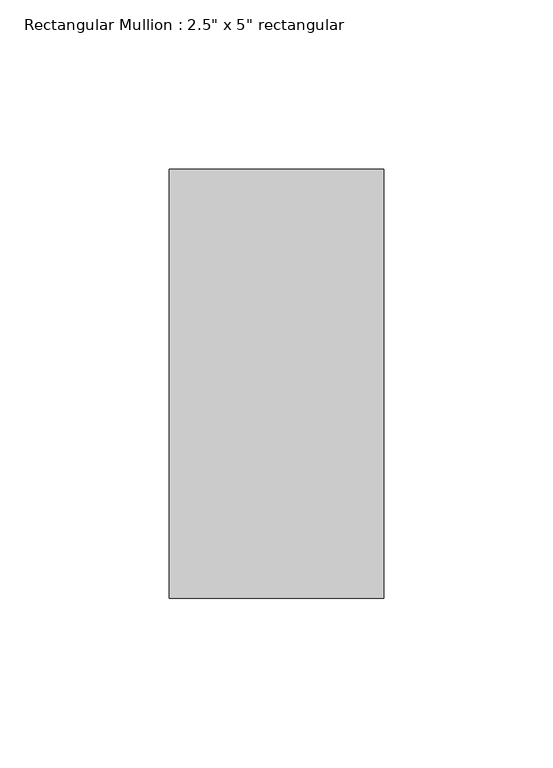
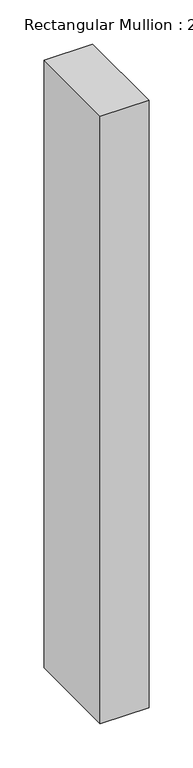
"""IFC4 building model written with IfcOpenShell, lengths in millimetres: member geometry."""

from ifc_helpers import new_model, si_unit, frame, origin, place, context, project, spatial, polyline, outline, extrude, source, transform, mapped, element, save


def member_86adc6a2(model_context):
    return source(origin(), model_context, "Body", "SweptSolid", [
        extrude(outline(polyline([(0.0, 63.5), (0.0, -63.5), (-63.5, -63.5), (-63.5, 63.5), (0.0, 63.5)])), frame((0.0, 0.0, -838.2), z_axis=(0.0, 0.0, 1.0), x_axis=(1.0, 0.0, 0.0)), (0.0, 0.0, 1.0), 838.2),
    ])


if __name__ == "__main__":
    model = new_model("IFC4")
    model_context = context("Model", 3, world=origin())
    ifc_project = project(units=[si_unit("LENGTHUNIT", "METRE", prefix="MILLI")], contexts=[model_context])
    site = spatial("IfcSite", under=ifc_project)
    building = spatial("IfcBuilding", under=site)
    placement = place(None, origin())
    member_shape = member_86adc6a2(model_context)
    element("IfcMember", 1, ObjectType="Rectangular Mullion : 2.5\" x 5\" rectangular", at=placement, inside=building, context=model_context, shape_type="MappedRepresentation", body=[
        mapped(member_shape, transform((0.0, 0.0, 0.0), x_axis=(1.0, 0.0, 0.0), y_axis=(0.0, 1.0, 0.0), z_axis=(0.0, 0.0, 1.0))),
    ])
    save(model, "model.ifc")

# Revit data of these elements
# Type "Rectangular Mullion : 2.5\" x 5\" rectangular"
#   built-in parameter 1007304 = 0.416667 (stored number, unit not read)
#   built-in parameter 1007301 = 0.104167 (stored number, unit not read)
#   built-in parameter 1007300 = 0.104167 (stored number, unit not read)
# Element 1 (IfcMember, "Rectangular Mullion : 2.5\" x 5\" rectangular")
#   Materials on its faces: "Aluminum"
# Materials
#   "Aluminum": class "Metal", colour RGB 247 247 247, transparency 0, Description = "Aluminum 6061", Cost = 0
